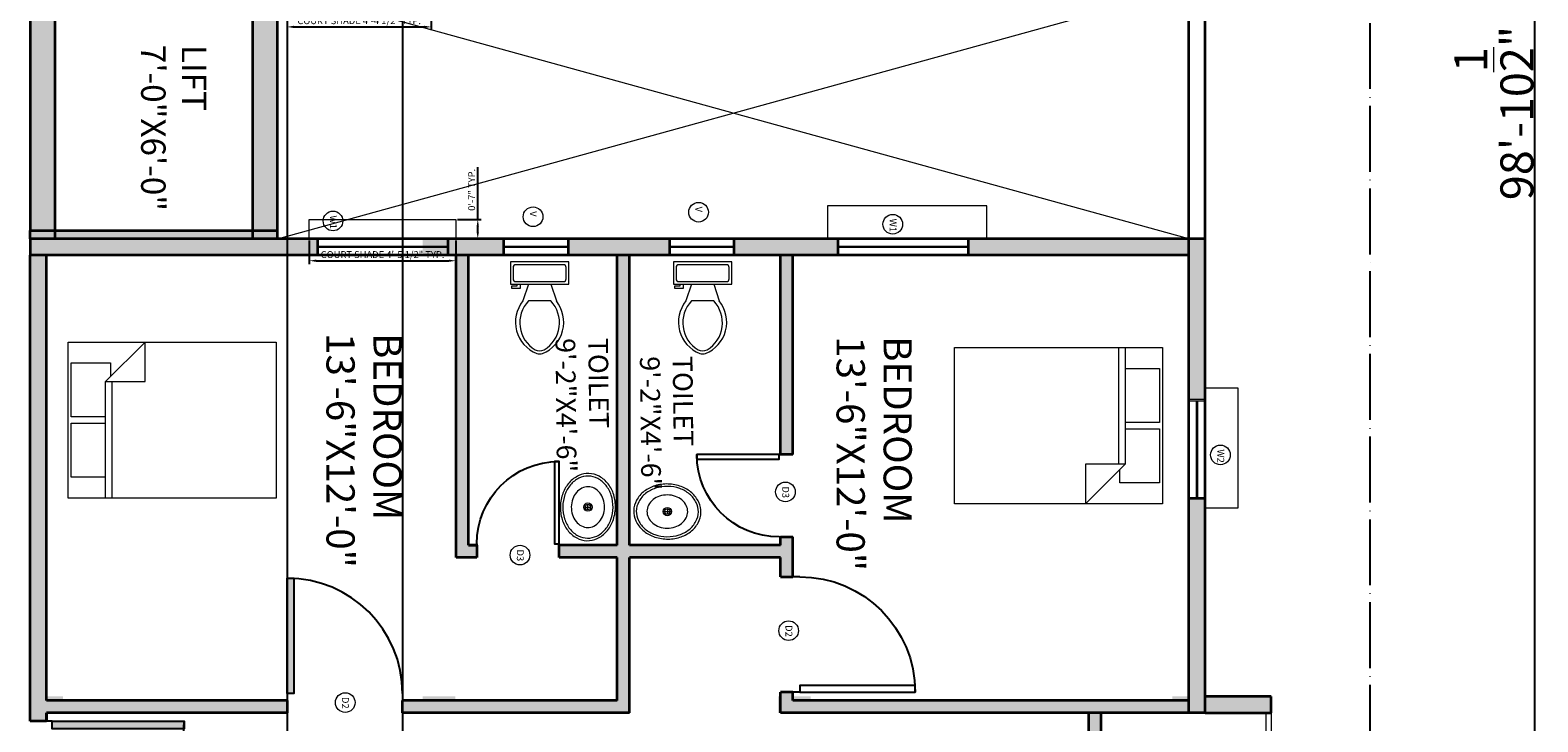
# Model space of a CAD drawing. Units: inches. Extents: x 7028582 to 7030319, y 63109697 to 63111305.
# Tile 13 of 18: x 7029748 to 7030297, y 63110278 to 63110530. Entities that reach past the tile are written whole.
import ezdxf

# ---------------------------------------------------------------- set-up
doc = ezdxf.new("R2010")
doc.units = ezdxf.units.IN
doc.linetypes.add('ACAD_ISO04W100', pattern=[30, 24, -3, 0, -3])
for name, color, linetype, lineweight in [('A-AREA-IDEN', 7, 'Continuous', 18), ('A-DOOR-IDEN', 20, 'Continuous', 13), ('A-FLOR-FIXT', 9, 'Continuous', 18), ('A-FLOR-HRAL', 5, 'Continuous', 18), ('A-FLOR-OPEN', 7, 'Continuous', 13), ('A-GLAZ-IDEN', 20, 'Continuous', 13), ('A-WALL-PATT', 8, 'Continuous', 13), ('C-ANNO-DIMS', 7, 'Continuous', 18), ('C-PROP', 1, 'ACAD_ISO04W100', 25), ('doors', 20, 'Continuous', 25), ('furniture', 9, 'Continuous', 18), ('S-COLS-PATT', 220, 'Continuous', 100), ('walls', 6, 'Continuous', 35), ('WINDOW SHADOW', 9, 'Continuous', 13), ('windows', 5, 'Continuous', 18)]:
    doc.layers.add(name, color=color, linetype=linetype, lineweight=lineweight)
doc.styles.get("Standard").update_dxf_attribs({"font": 'arial.ttf'})
doc.dimstyles.new('ISO-25', dxfattribs={"dimtxt": 2.5, "dimasz": 2.5, "dimexe": 1.25, "dimexo": 0.625, "dimtad": 1, "dimlunit": 4, "dimtxsty": 'Standard', "dimcen": 2.5, "dimadec": 0, "dimazin": 0, "dimtfac": 1, "dimtmove": 0, "dimatfit": 3, "dimfxl": 1, "dimarcsym": 0})

# ---------------------------------------------------------------- blocks, each defined once
blk = doc.blocks.new('*U2')
for p, q in [((0, 0), (0, -5)), ((30, 0), (30, -5))]:
    blk.add_line(p, q)
blk.add_lwpolyline([(0, 0), (0, 30), (1.75, 30), (1.75, 0)], close=True)
blk.add_arc((0, 0), 30, 0, 90)
blk = doc.blocks.new('Toilet - top')
for p, q in [((9.5, -6), (9.5, -2)), ((-10, -8.5), (-8, -8.5)), ((-10, -9.5), (-10, -8.5)), ((-7, -9.5), (-10, -9.5)), ((-8, -8.5), (-8, -8)), ((-7, -8), (-7, -9.5)), ((-4, -8), (-6, -14)), ((4, -8), (6, -14)), ((4, -14), (-4, -14))]:
    blk.add_line(p, q)
blk.add_lwpolyline([(10.5, -8), (10.5, 0), (-10.5, 0), (-10.5, -8)], close=True)
for points in [[(-9.5, -2), (-9.5, -6)], [(8.5, -1), (-8.5, -1)], [(-8.5, -7), (8.5, -7)]]:
    blk.add_lwpolyline(points)
for centre, radius, start, end in [((-8.62, -1.88), 0.884, 81.8699, 188.1301), ((8.62, -1.88), 0.884, 351.8699, 98.1301), ((-8.62, -6.12), 0.884, 171.8699, 278.1301), ((8.62, -6.12), 0.884, 261.8699, 8.1301), ((3.52, -21.58), 12.17, 141.4691, 247.9714), ((4.2, -21.82), 11.33, 136.3677, 238.9468), ((-3.52, -21.58), 12.17, 292.0284, 38.5307), ((-4.2, -21.82), 11.33, 301.053, 43.6321), ((0, -27.88), 4, 245.7318, 294.2682), ((0, -29), 4, 254.8605, 285.1395)]:
    blk.add_arc(centre, radius, start, end)
blk = doc.blocks.new('Sink - Oval top')
for p, q in [((-1, 0), (1, 0)), ((0, 1), (0, -1))]:
    blk.add_line(p, q)
for points in [[(-12.23, 0.39, 0.117634), (-11.46, -3.36, 0.104469), (-8.88, -6.8, 0.090016), (-5.08, -9.07, 0.08192), (-0.32, -10.02, 0.08192), (4.49, -9.38, 0.090016), (8.42, -7.36, 0.104469), (11.22, -4.09, 0.117634), (12.23, -0.39, 0.117634), (11.46, 3.36, 0.104469), (8.88, 6.8, 0.090016), (5.08, 9.07, 0.08192), (0.32, 10.02, 0.08192), (-4.49, 9.38, 0.090016), (-8.42, 7.36, 0.104469), (-11.22, 4.09, 0.117634)], [(-11.29, 0.16, 0.118622), (-10.52, -3.25, 0.104678), (-8.07, -6.36, 0.089562), (-4.54, -8.37, 0.081185), (-0.13, -9.15, 0.081185), (4.3, -8.49, 0.089562), (7.89, -6.58, 0.104678), (10.42, -3.55, 0.118622), (11.29, -0.16, 0.118622), (10.52, 3.25, 0.104678), (8.07, 6.36, 0.089562), (4.54, 8.37, 0.081185), (0.13, 9.15, 0.081185), (-4.3, 8.49, 0.089562), (-7.89, 6.58, 0.104678), (-10.42, 3.55, 0.118622)], [(-7.42, 0.08, 0.118283), (-6.91, -2.17, 0.104607), (-5.29, -4.21, 0.089718), (-2.97, -5.53, 0.081436), (-0.07, -6.04, 0.081436), (2.84, -5.59, 0.089718), (5.2, -4.33, 0.104607), (6.86, -2.32, 0.118283), (7.42, -0.08, 0.118283), (6.91, 2.17, 0.104607), (5.29, 4.21, 0.089718), (2.97, 5.53, 0.081436), (0.07, 6.04, 0.081436), (-2.84, 5.59, 0.089718), (-5.2, 4.33, 0.104607), (-6.86, 2.32, 0.118283)]]:
    blk.add_lwpolyline(points, format="xyb", close=True)
for radius in [1.5, 1]:
    blk.add_circle((0, 0), radius)
blk = doc.blocks.new('Bed - Queen')
for p, q in [((0, -80.00003), (0, 0)), ((0, 0), (59.99999, 0)), ((59.99999, 0), (59.99999, -80.00003)), ((7.99999, -1.2), (28.79998, -1.2)), ((7.99999, -14.4), (7.99999, -1.2)), ((28.79998, -1.2), (28.79998, -14.4)), ((31.19999, -1.2), (51.99999, -1.2)), ((31.19999, -14.4), (31.19999, -1.2)), ((51.99999, -1.2), (51.99999, -16.4)), ((0, -14.4), (44.8, -14.4)), ((44.8, -16.8), (0, -16.8)), ((59.99999, -29.6), (44.8, -14.4)), ((44.8, -14.4), (44.8, -29.6)), ((51.99999, -16.4), (46.79936, -16.4)), ((44.8, -29.6), (59.99999, -29.6)), ((59.99999, -80.00003), (0, -80.00003))]:
    blk.add_line(p, q)
blk = doc.blocks.new('*D10')
at = {"layer": 'C-ANNO-DIMS', "color": 0, "lineweight": -2, "transparency": 16777216}
for p, q in [((7030236.33, 63111093.06), (7030296.71, 63111093.06)), ((7030295.46, 63111090.56), (7030295.46, 63109909.06)), ((7030236.33, 63109906.56), (7030296.71, 63109906.56))]:
    blk.add_line(p, q, dxfattribs=at)
at = {"layer": 'C-ANNO-DIMS', "color": 0, "lineweight": 100, "transparency": 16777216}
for points in [[(7030295.04, 63111090.56), (7030295.88, 63111090.56), (7030295.46, 63111093.06)], [(7030295.04, 63109909.06), (7030295.88, 63109909.06), (7030295.46, 63109906.56)]]:
    blk.add_solid(points, dxfattribs=at)
at = {"layer": 'Defpoints', "color": 0, "lineweight": 100, "transparency": 16777216}
for p in [(7030235.71, 63111093.06), (7030235.71, 63109906.56), (7030295.46, 63109906.56)]:
    blk.add_point(p, dxfattribs=at)
at = {"layer": 'C-ANNO-DIMS', "color": 0, "transparency": 16777216, "insert": (7030280.69, 63110499.81), "char_height": 12, "attachment_point": 5, "rotation": 90}
blk.add_mtext('98\'-10{\\H1x;\\S1/2;}"', dxfattribs=at)
blk = doc.blocks.new('WIN-SASH-36')
for p, q in [((0, 36.05), (0, 0)), ((6, 35.55), (0, 35.55)), ((2.8, 35.55), (2.8, 0.5)), ((3.2, 35.55), (3.2, 0.5)), ((6, 0), (6, 36.05)), ((0, 0.5), (6, 0.5))]:
    blk.add_line(p, q)
blk = doc.blocks.new('WIN-SASH-24')
for p, q in [((24.05, 6), (0, 6)), ((0.5, 6), (0.5, 0)), ((23.55, 0), (23.55, 6)), ((0, 0), (24.05, 0)), ((23.55, 3.2), (0.5, 3.2)), ((23.55, 2.8), (0.5, 2.8))]:
    blk.add_line(p, q)
blk = doc.blocks.new('WIN-SASH-48')
for p, q in [((48.05, 6), (0, 6)), ((0.5, 6), (0.5, 0)), ((47.55, 0), (47.55, 6)), ((47.55, 3.2), (0.5, 3.2)), ((47.55, 2.8), (0.5, 2.8)), ((0, 0), (48.05, 0))]:
    blk.add_line(p, q)
blk = doc.blocks.new('WINDOW-SHADE-SIDE-44')
for p, q in [((12, 43.55), (0, 43.55)), ((12, 0), (12, 43.55)), ((0, 0), (12, 0))]:
    blk.add_line(p, q)
blk = doc.blocks.new('WINDOW-SHADE-HEAD-58')
for p, q in [((57.96, 12), (0, 12)), ((0, 12), (0, 0)), ((57.96, 0), (57.96, 12))]:
    blk.add_line(p, q)
blk = doc.blocks.new('WINDOW-SHADE-COURT-53')
for p, q in [((0, 0), (0, 7.06)), ((0, 7.06), (53.29, 7.06)), ((53.29, 7.06), (53.29, 0))]:
    blk.add_line(p, q)
blk = doc.blocks.new('BALCONY-GUARD-12FT')
for p, q in [((0, 144), (0, 0)), ((2, 144), (2, 0))]:
    blk.add_line(p, q)
blk = doc.blocks.new('TAG-D2-MT-R')
blk.add_circle((3.58, 3.58), 3.58)
at = {"insert": (4.93, 5.6), "char_height": 2.5, "attachment_point": 1, "rotation": 270}
blk.add_mtext_dynamic_manual_height_columns('D2', width=2.5021, gutter_width=12.5, heights=[0], dxfattribs=at)
blk = doc.blocks.new('TAG-D3-MT-R')
blk.add_circle((3.58, 3.58), 3.58)
at = {"insert": (4.93, 5.6), "char_height": 2.5, "attachment_point": 1, "rotation": 270}
blk.add_mtext_dynamic_manual_height_columns('D3', width=2.5021, gutter_width=12.5, heights=[0], dxfattribs=at)
blk = doc.blocks.new('TAG-V-MT-R')
blk.add_circle((3.58, 3.58), 3.58)
at = {"insert": (4.93, 5.6), "char_height": 2.5, "attachment_point": 1, "rotation": 270}
blk.add_mtext_dynamic_manual_height_columns('V', width=2.5021, gutter_width=12.5, heights=[0], dxfattribs=at)
blk = doc.blocks.new('TAG-W1-MT-R')
blk.add_circle((3.58, 3.58), 3.58)
at = {"insert": (4.93, 5.6), "char_height": 2.5, "attachment_point": 1, "rotation": 270}
blk.add_mtext_dynamic_manual_height_columns('W1', width=2.5021, gutter_width=12.5, heights=[0], dxfattribs=at)
blk = doc.blocks.new('TAG-W2-MT-R')
blk.add_circle((3.58, 3.58), 3.58)
at = {"insert": (4.93, 5.6), "char_height": 2.5, "attachment_point": 1, "rotation": 270}
blk.add_mtext_dynamic_manual_height_columns('W2', width=2.5021, gutter_width=12.5, heights=[0], dxfattribs=at)
blk = doc.blocks.new('*D95')
at = {"layer": 'C-ANNO-DIMS', "color": 0, "lineweight": -2, "transparency": 16777216}
for p, q in [((7029841.67, 63110538.39), (7029841.67, 63110529.9)), ((7029894.13, 63110538.39), (7029894.13, 63110529.9)), ((7029844.17, 63110531.15), (7029891.63, 63110531.15))]:
    blk.add_line(p, q, dxfattribs=at)
at = {"layer": 'C-ANNO-DIMS', "color": 0, "lineweight": 100, "transparency": 16777216}
for points in [[(7029844.17, 63110531.56), (7029844.17, 63110530.73), (7029841.67, 63110531.15)], [(7029891.63, 63110531.56), (7029891.63, 63110530.73), (7029894.13, 63110531.15)]]:
    blk.add_solid(points, dxfattribs=at)
at = {"layer": 'Defpoints', "color": 0, "lineweight": 100, "transparency": 16777216}
for p in [(7029841.67, 63110539.02), (7029894.13, 63110539.02), (7029894.13, 63110531.15)]:
    blk.add_point(p, dxfattribs=at)
at = {"layer": 'C-ANNO-DIMS', "color": 0, "transparency": 16777216, "insert": (7029867.9, 63110533.07), "char_height": 2.5, "attachment_point": 5}
blk.add_mtext('COURT SHADE 4\'-4 1/2" TYP.', dxfattribs=at)
blk = doc.blocks.new('*D97')
at = {"layer": 'C-ANNO-DIMS', "color": 0, "lineweight": -2, "transparency": 16777216}
for p, q in [((7029849.76, 63110453.43), (7029849.76, 63110444.81)), ((7029903.05, 63110453.43), (7029903.05, 63110444.81)), ((7029852.26, 63110446.06), (7029900.55, 63110446.06))]:
    blk.add_line(p, q, dxfattribs=at)
at = {"layer": 'C-ANNO-DIMS', "color": 0, "lineweight": 100, "transparency": 16777216}
for points in [[(7029852.26, 63110446.48), (7029852.26, 63110445.65), (7029849.76, 63110446.06)], [(7029900.55, 63110446.48), (7029900.55, 63110445.65), (7029903.05, 63110446.06)]]:
    blk.add_solid(points, dxfattribs=at)
at = {"layer": 'Defpoints', "color": 0, "lineweight": 100, "transparency": 16777216}
for p in [(7029849.76, 63110454.06), (7029903.05, 63110454.06), (7029903.05, 63110446.06)]:
    blk.add_point(p, dxfattribs=at)
at = {"layer": 'C-ANNO-DIMS', "color": 0, "transparency": 16777216, "insert": (7029876.41, 63110447.98), "char_height": 2.5, "attachment_point": 5}
blk.add_mtext('COURT SHADE 4\'-5 1/2" TYP.', dxfattribs=at)
blk = doc.blocks.new('*D98')
at = {"layer": 'C-ANNO-DIMS', "color": 0, "lineweight": -2, "transparency": 16777216}
for p, q in [((7029911.05, 63110461.12), (7029911.05, 63110480.1)), ((7029903.68, 63110461.12), (7029912.3, 63110461.12)), ((7029911.05, 63110456.56), (7029911.05, 63110458.62)), ((7029903.68, 63110454.06), (7029912.3, 63110454.06))]:
    blk.add_line(p, q, dxfattribs=at)
at = {"layer": 'C-ANNO-DIMS', "color": 0, "lineweight": 100, "transparency": 16777216}
for points in [[(7029910.63, 63110458.62), (7029911.46, 63110458.62), (7029911.05, 63110461.12)], [(7029910.63, 63110456.56), (7029911.46, 63110456.56), (7029911.05, 63110454.06)]]:
    blk.add_solid(points, dxfattribs=at)
at = {"layer": 'Defpoints', "color": 0, "lineweight": 100, "transparency": 16777216}
for p in [(7029903.05, 63110461.12), (7029911.05, 63110461.12), (7029903.05, 63110454.06)]:
    blk.add_point(p, dxfattribs=at)
at = {"layer": 'C-ANNO-DIMS', "color": 0, "transparency": 16777216, "insert": (7029909.15, 63110471.86), "char_height": 2.5, "attachment_point": 5, "rotation": 90}
blk.add_mtext('0\'-7" TYP.', dxfattribs=at)
blk = doc.blocks.new('*D105')
at = {"layer": 'C-ANNO-DIMS', "color": 0, "lineweight": -2, "transparency": 16777216}
for p, q in [((7029841.68, 63110859.93), (7029841.68, 63109697.14)), ((7029883.68, 63110859.93), (7029883.68, 63109697.14)), ((7029844.18, 63109698.39), (7029881.18, 63109698.39))]:
    blk.add_line(p, q, dxfattribs=at)
at = {"layer": 'C-ANNO-DIMS', "color": 0, "lineweight": 100, "transparency": 16777216}
for points in [[(7029844.18, 63109698.8), (7029844.18, 63109697.97), (7029841.68, 63109698.39)], [(7029881.18, 63109698.8), (7029881.18, 63109697.97), (7029883.68, 63109698.39)]]:
    blk.add_solid(points, dxfattribs=at)
at = {"layer": 'Defpoints', "color": 0, "lineweight": 100, "transparency": 16777216}
for p in [(7029841.68, 63110860.56), (7029883.68, 63110860.56), (7029883.68, 63109698.39)]:
    blk.add_point(p, dxfattribs=at)
at = {"layer": 'C-ANNO-DIMS', "color": 0, "transparency": 16777216, "insert": (7029862.68, 63109700.29), "char_height": 2.5, "attachment_point": 5}
blk.add_mtext('3\'-6"', dxfattribs=at)

msp = doc.modelspace()

# ---------------------------------------------------------------- hatches: boundary and pattern name
at = {"layer": 'A-WALL-PATT'}
h = msp.add_hatch(color=256, dxfattribs=at)
h.dxf.hatch_style = 1
h.paths.add_polyline_path([(7029757.205, 63110542.557), (7029748.205, 63110542.557), (7029748.205, 63110457.057), (7029757.205, 63110457.057)])
h = msp.add_hatch(color=256, dxfattribs=at)
h.dxf.hatch_style = 1
h.paths.add_polyline_path([(7029838.205, 63110542.557), (7029829.205, 63110542.557), (7029829.205, 63110457.057), (7029838.205, 63110457.057)])
h = msp.add_hatch(color=256, dxfattribs=at)
h.dxf.hatch_style = 1
h.paths.add_polyline_path([(7029757.205, 63110457.057), (7029748.205, 63110457.057), (7029748.205, 63110454.057), (7029757.205, 63110454.057)])
h = msp.add_hatch(color=256, dxfattribs=at)
h.dxf.hatch_style = 1
h.paths.add_polyline_path([(7029748.205, 63110454.057), (7029748.205, 63110448.057), (7029852.47, 63110448.057), (7029852.47, 63110454.057), (7029825.251, 63110454.057)])
h = msp.add_hatch(color=256, dxfattribs=at)
h.dxf.hatch_style = 1
h.paths.add_polyline_path([(7029852.47, 63110454.057), (7029825.251, 63110454.057), (7029748.205, 63110454.057), (7029748.205, 63110448.057), (7029852.47, 63110448.057)])
h = msp.add_hatch(color=256, dxfattribs=at)
h.dxf.hatch_style = 1
h.paths.add_polyline_path([(7029829.205, 63110457.057), (7029757.205, 63110457.057), (7029757.205, 63110454.057), (7029825.251, 63110454.057), (7029829.205, 63110454.057)])
h = msp.add_hatch(color=256, dxfattribs=at)
h.dxf.hatch_style = 1
h.paths.add_polyline_path([(7029838.205, 63110457.057), (7029829.205, 63110457.057), (7029829.205, 63110454.057), (7029838.205, 63110454.057)])
h = msp.add_hatch(color=256, dxfattribs=at)
h.dxf.hatch_style = 1
h.paths.add_polyline_path([(7029900.518, 63110448.057), (7029920.21, 63110448.057), (7029920.21, 63110454.057), (7029900.518, 63110454.057)])
h = msp.add_hatch(color=256, dxfattribs=at)
h.dxf.hatch_style = 1
h.paths.add_polyline_path([(7029980.53, 63110454.057), (7029944.258, 63110454.057), (7029944.258, 63110448.057), (7029980.53, 63110448.057)])
h = msp.add_hatch(color=256, dxfattribs=at)
h.dxf.hatch_style = 1
h.paths.add_polyline_path([(7030041.813, 63110454.057), (7030004.578, 63110454.057), (7030004.578, 63110448.057), (7030041.813, 63110448.057)])
h.paths.add_polyline_path([(7030025.705, 63110448.057), (7030021.205, 63110448.057), (7030021.205, 63110375.557), (7030025.705, 63110375.557)], flags=0)
h = msp.add_hatch(color=256, dxfattribs=at)
h.dxf.hatch_style = 1
h.paths.add_polyline_path([(7030175.705, 63110454.057), (7030089.861, 63110454.057), (7030089.861, 63110448.057), (7030169.705, 63110448.057), (7030169.705, 63110395.515), (7030175.705, 63110395.515)])
h = msp.add_hatch(color=256, dxfattribs=at)
h.dxf.hatch_style = 1
h.paths.add_polyline_path([(7029754.205, 63110278.557), (7029756.205, 63110278.557), (7029804.205, 63110278.557), (7029804.205, 63110275.757), (7029756.205, 63110275.757), (7029756.205, 63110278.557), (7029748.205, 63110278.557), (7029748.205, 63110448.057), (7029754.205, 63110448.057), (7029754.205, 63110286.057), (7029841.685, 63110286.057), (7029841.685, 63110288.557), (7029841.685, 63110330.557), (7029844.135, 63110330.557), (7029844.135, 63110288.557), (7029841.685, 63110288.557), (7029841.685, 63110281.557), (7029754.205, 63110281.557)])
h = msp.add_hatch(color=256, dxfattribs=at)
h.dxf.hatch_style = 1
h.paths.add_polyline_path([(7030025.705, 63110448.057), (7030021.205, 63110448.057), (7030021.205, 63110375.557), (7030025.705, 63110375.557)], flags=0)
h.paths.add_polyline_path([(7030025.705, 63110345.557), (7030021.205, 63110345.557), (7030021.205, 63110342.557), (7029966.205, 63110342.557), (7029966.205, 63110448.057), (7029961.705, 63110448.057), (7029961.705, 63110342.557), (7029940.705, 63110342.557), (7029940.705, 63110338.057), (7029961.705, 63110338.057), (7029961.705, 63110286.057), (7029883.685, 63110286.057), (7029883.685, 63110281.557), (7029966.205, 63110281.557), (7029966.205, 63110338.057), (7030021.205, 63110338.057), (7030021.205, 63110331.057), (7030025.705, 63110331.057)])
h = msp.add_hatch(color=256, dxfattribs=at)
h.dxf.hatch_style = 1
h.paths.add_polyline_path([(7029907.705, 63110448.057), (7029903.205, 63110448.057), (7029903.205, 63110338.057), (7029910.705, 63110338.057), (7029910.705, 63110342.557), (7029907.705, 63110342.557)], flags=17)
h = msp.add_hatch(color=256, dxfattribs=at)
h.dxf.hatch_style = 1
h.paths.add_polyline_path([(7030025.705, 63110448.057), (7030021.205, 63110448.057), (7030021.205, 63110375.557), (7030025.705, 63110375.557)])
h = msp.add_hatch(color=256, dxfattribs=at)
h.dxf.hatch_style = 1
h.paths.add_polyline_path([(7030175.705, 63110359.466), (7030169.705, 63110359.466), (7030169.705, 63110281.557), (7030175.705, 63110281.557)])
h = msp.add_hatch(color=256, dxfattribs=at)
h.dxf.hatch_style = 1
h.paths.add_polyline_path([(7030169.705, 63110286.057), (7030025.705, 63110286.057), (7030025.705, 63110289.057), (7030021.205, 63110289.057), (7030021.205, 63110281.557), (7030169.705, 63110281.557)])
h = msp.add_hatch(color=256, dxfattribs=at)
h.dxf.hatch_style = 1
h.paths.add_polyline_path([(7030199.705, 63110287.557), (7030175.705, 63110287.557), (7030175.705, 63110281.557), (7030199.705, 63110281.557)])
h = msp.add_hatch(color=256, dxfattribs=at)
h.dxf.hatch_style = 1
h.paths.add_polyline_path([(7030137.705, 63110281.557), (7030133.205, 63110281.557), (7030133.205, 63110243.163), (7030137.705, 63110243.163)])
at = {"layer": 'S-COLS-PATT'}
h = msp.add_hatch(color=256, dxfattribs=at)
h.dxf.hatch_style = 1
h.paths.add_polyline_path([(7029760.108, 63110454.057), (7029748.205, 63110454.057), (7029748.205, 63110448.057), (7029760.108, 63110448.057)])
h = msp.add_hatch(color=256, dxfattribs=at)
h.dxf.hatch_style = 1
h.paths.add_polyline_path([(7029902.915, 63110454.057), (7029891, 63110454.057), (7029891, 63110448.057), (7029902.915, 63110448.057)])
h = msp.add_hatch(color=256, dxfattribs=at)
h.dxf.hatch_style = 1
h.paths.add_polyline_path([(7030032.194, 63110454.057), (7030020.279, 63110454.057), (7030020.279, 63110448.057), (7030032.194, 63110448.057)])
h = msp.add_hatch(color=256, dxfattribs=at)
h.dxf.hatch_style = 1
h.paths.add_polyline_path([(7030175.705, 63110454.057), (7030163.791, 63110454.057), (7030163.791, 63110448.057), (7030175.705, 63110448.057)])
h = msp.add_hatch(color=256, dxfattribs=at)
h.dxf.hatch_style = 1
h.paths.add_polyline_path([(7029760.108, 63110287.557), (7029748.205, 63110287.557), (7029748.205, 63110281.557), (7029760.108, 63110281.557)])
h = msp.add_hatch(color=256, dxfattribs=at)
h.dxf.hatch_style = 1
h.paths.add_polyline_path([(7029902.915, 63110287.557), (7029891, 63110287.557), (7029891, 63110281.557), (7029902.915, 63110281.557)])
h = msp.add_hatch(color=256, dxfattribs=at)
h.dxf.hatch_style = 1
h.paths.add_polyline_path([(7030032.194, 63110287.557), (7030020.279, 63110287.557), (7030020.279, 63110281.557), (7030032.194, 63110281.557)])
h = msp.add_hatch(color=256, dxfattribs=at)
h.dxf.hatch_style = 1
h.paths.add_polyline_path([(7030175.705, 63110287.557), (7030163.791, 63110287.557), (7030163.791, 63110281.557), (7030175.705, 63110281.557)])

# ---------------------------------------------------------------- linework, layer by layer
at = {"layer": 'A-FLOR-OPEN'}
for p, q in [((7030169.705, 63110454.057), (7029838.205, 63110545.557)), ((7029838.205, 63110454.057), (7030169.705, 63110545.557))]:
    msp.add_line(p, q, dxfattribs=at)
at = {"layer": 'C-PROP'}
msp.add_line((7030235.705, 63109906.557), (7030235.705, 63111093.057), dxfattribs=at)
at = {"layer": 'walls'}
for p, q in [((7030175.705, 63110281.557), (7030175.705, 63110716.557)), ((7029748.205, 63110542.557), (7029748.205, 63110457.057)), ((7029757.205, 63110545.557), (7029757.205, 63110454.057)), ((7029829.205, 63110454.057), (7029829.205, 63110545.557)), ((7029838.205, 63110454.057), (7029838.205, 63110545.557)), ((7030169.705, 63110281.557), (7030169.705, 63110545.557)), ((7029748.205, 63110454.057), (7029748.205, 63110457.057)), ((7029748.205, 63110457.057), (7029757.205, 63110457.057)), ((7029825.251, 63110454.057), (7029748.205, 63110454.057)), ((7029748.205, 63110454.057), (7029748.205, 63110448.057)), ((7029757.205, 63110457.057), (7029829.205, 63110457.057)), ((7030175.705, 63110454.057), (7029825.251, 63110454.057)), ((7029829.205, 63110457.057), (7029838.205, 63110457.057)), ((7030175.705, 63110281.557), (7030175.705, 63110454.057)), ((7029748.205, 63110278.557), (7029748.205, 63110448.057)), ((7030169.705, 63110448.057), (7029748.205, 63110448.057)), ((7029754.205, 63110286.057), (7029754.205, 63110448.057)), ((7029903.205, 63110338.057), (7029903.205, 63110448.057)), ((7029907.705, 63110342.557), (7029907.705, 63110448.057)), ((7029961.705, 63110342.557), (7029961.705, 63110448.057)), ((7029966.205, 63110342.557), (7029966.205, 63110448.057)), ((7030021.205, 63110375.557), (7030021.205, 63110448.057)), ((7030025.705, 63110375.557), (7030025.705, 63110448.057)), ((7030169.705, 63110281.557), (7030169.705, 63110448.057)), ((7030025.705, 63110375.557), (7030021.205, 63110375.557)), ((7030021.205, 63110342.557), (7030021.205, 63110345.557)), ((7030021.205, 63110342.557), (7030021.205, 63110345.557)), ((7030021.205, 63110345.557), (7030025.705, 63110345.557)), ((7030025.705, 63110331.057), (7030025.705, 63110345.557)), ((7029910.705, 63110338.057), (7029903.205, 63110338.057)), ((7029910.705, 63110342.557), (7029907.705, 63110342.557)), ((7029907.705, 63110342.557), (7029910.705, 63110342.557)), ((7029910.705, 63110342.557), (7029910.705, 63110338.057)), ((7029961.705, 63110342.557), (7029940.705, 63110342.557)), ((7029940.705, 63110338.057), (7029940.705, 63110342.557)), ((7029961.705, 63110338.057), (7029940.705, 63110338.057)), ((7029961.705, 63110286.057), (7029961.705, 63110338.057)), ((7030021.205, 63110342.557), (7029966.205, 63110342.557)), ((7029966.205, 63110281.557), (7029966.205, 63110338.057)), ((7030021.205, 63110338.057), (7029966.205, 63110338.057)), ((7030021.205, 63110331.057), (7030021.205, 63110338.057)), ((7030021.205, 63110331.057), (7030025.705, 63110331.057)), ((7030021.205, 63110281.557), (7030021.205, 63110289.057)), ((7030025.705, 63110289.057), (7030021.205, 63110289.057)), ((7030025.705, 63110286.057), (7030025.705, 63110289.057)), ((7030025.705, 63110286.057), (7030025.705, 63110289.057)), ((7029841.685, 63110286.057), (7029754.205, 63110286.057)), ((7029841.685, 63110286.057), (7029841.685, 63110281.557)), ((7029883.685, 63110281.557), (7029883.685, 63110286.057)), ((7029961.705, 63110286.057), (7029883.685, 63110286.057)), ((7030169.705, 63110286.057), (7030025.705, 63110286.057)), ((7030199.705, 63110287.557), (7030175.705, 63110287.557)), ((7030199.705, 63110281.557), (7030199.705, 63110287.557)), ((7029754.205, 63110278.557), (7029748.205, 63110278.557)), ((7029754.205, 63110278.557), (7029754.205, 63110281.557)), ((7029841.685, 63110281.557), (7029754.205, 63110281.557)), ((7029754.205, 63110281.557), (7029754.205, 63110278.557)), ((7029966.205, 63110281.557), (7029883.685, 63110281.557)), ((7030175.705, 63110281.557), (7030021.205, 63110281.557)), ((7030133.205, 63110281.557), (7030133.205, 63110137.557)), ((7030137.705, 63110281.557), (7030137.705, 63110137.557)), ((7030175.705, 63110281.557), (7030199.705, 63110281.557))]:
    msp.add_line(p, q, dxfattribs=at)
at = {"layer": 'windows'}
for p, q in [((7029852.47, 63110454.057), (7029852.47, 63110448.057)), ((7029900.518, 63110448.057), (7029900.518, 63110454.057)), ((7029920.21, 63110454.057), (7029920.21, 63110448.057)), ((7029944.258, 63110448.057), (7029944.258, 63110454.057)), ((7029980.53, 63110454.057), (7029980.53, 63110448.057)), ((7030004.578, 63110448.057), (7030004.578, 63110454.057)), ((7030041.813, 63110454.057), (7030041.813, 63110448.057)), ((7030089.861, 63110448.057), (7030089.861, 63110454.057)), ((7030175.776, 63110395.515), (7030169.776, 63110395.515)), ((7030169.776, 63110359.466), (7030175.776, 63110359.466))]:
    msp.add_line(p, q, dxfattribs=at)

# ---------------------------------------------------------------- block references
at = {"layer": 'A-DOOR-IDEN'}
for name, p in [('TAG-D3-MT-R', (7030019.402, 63110358.359)), ('TAG-D3-MT-R', (7029922.838, 63110335.381)), ('TAG-D2-MT-R', (7030020.567, 63110307.879)), ('TAG-D2-MT-R', (7029859.234, 63110281.722))]:
    msp.add_blockref(name, p, dxfattribs=at)
at = {"layer": 'A-FLOR-FIXT', "xscale": 1.013555723357934, "yscale": 1.013555723357934, "zscale": 1.013555723357934}
for p in [(7029933.551, 63110445.605), (7029992.842, 63110445.605)]:
    msp.add_blockref('Toilet - top', p, dxfattribs=at)
at = {"layer": 'A-FLOR-FIXT', "rotation": 90}
msp.add_blockref('Sink - Oval top', (7029951.122, 63110356.416), dxfattribs=at)
at = {"layer": 'A-FLOR-FIXT'}
msp.add_blockref('Sink - Oval top', (7029980.015, 63110354.801), dxfattribs=at)
at = {"layer": 'A-FLOR-HRAL'}
msp.add_blockref('BALCONY-GUARD-12FT', (7030197.705, 63110137.557), dxfattribs=at)
at = {"layer": 'A-GLAZ-IDEN'}
for name, p in [('TAG-W1-MT-R', (7029854.806, 63110456.953)), ('TAG-V-MT-R', (7029927.584, 63110458.489)), ('TAG-V-MT-R', (7029987.808, 63110460.151)), ('TAG-W1-MT-R', (7030058.467, 63110455.779)), ('TAG-W2-MT-R', (7030177.672, 63110371.827))]:
    msp.add_blockref(name, p, dxfattribs=at)
at = {"layer": 'doors', "xscale": -1}
msp.add_blockref('*U2', (7029940.705, 63110343.057), dxfattribs=at)
at = {"layer": 'doors', "xscale": -1, "rotation": 90}
msp.add_blockref('*U2', (7030020.705, 63110375.557), dxfattribs=at)
at = {"layer": 'doors', "xscale": 1.399999999999999, "yscale": 1.399999999999999, "zscale": 1.399999999999999}
msp.add_blockref('*U2', (7029841.685, 63110288.557), dxfattribs=at)
at = {"layer": 'doors', "rotation": 270}
for p, xscale, yscale, zscale in [((7030028.205, 63110289.057), -1.399999999999999, 1.399999999999999, 1.399999999999999), ((7029756.205, 63110278.557), 1.599999999999999, 1.599999999999999, 1.599999999999999)]:
    msp.add_blockref('*U2', p, dxfattribs=dict(at, xscale=xscale, yscale=yscale, zscale=zscale))
at = {"layer": 'furniture', "xscale": 0.9464141645025947, "yscale": 0.9464141645025947, "zscale": 0.9464141645025947}
for p, rotation in [((7029761.974, 63110359.688), 89.99999999999999), ((7030160.206, 63110414.435), 270)]:
    msp.add_blockref('Bed - Queen', p, dxfattribs=dict(at, rotation=rotation))
at = {"layer": 'WINDOW SHADOW'}
for name, p in [('WINDOW-SHADE-HEAD-58', (7030038.324, 63110454.057)), ('WINDOW-SHADE-COURT-53', (7029849.762, 63110454.057)), ('WINDOW-SHADE-SIDE-44', (7030175.705, 63110356.171))]:
    msp.add_blockref(name, p, dxfattribs=at)
at = {"layer": 'windows'}
for name, p in [('WIN-SASH-48', (7029852.47, 63110448.057)), ('WIN-SASH-24', (7029920.21, 63110448.057)), ('WIN-SASH-24', (7029980.53, 63110448.057)), ('WIN-SASH-48', (7030041.813, 63110448.057))]:
    msp.add_blockref(name, p, dxfattribs=at)
at = {"layer": 'windows', "rotation": 180}
msp.add_blockref('WIN-SASH-36', (7030175.776, 63110395.515), dxfattribs=at)

# ---------------------------------------------------------------- texts
at = {"layer": 'A-AREA-IDEN', "attachment_point": 1}
for s, width, gutter_width, insert, char_height, rotation in [('LIFT\\P7\'-0"X6\'-0"', 27.37587, 44.409, (7029812.273, 63110524.612), 8.88185, 270), ('BEDROOM\\P13\'-6"X12\'-0"', 82.04322, 51.315, (7029883.378, 63110419.737), 10.26307, 270), ('TOILET\\P9\'-2"X4\'-6"', 42.97461, 35.821, (7029958.409, 63110418.065), 7.16426, 270.6464), ('BEDROOM\\P13\'-6"X12\'-0"', 82.04322, 51.315, (7030068.956, 63110418.575), 10.26307, 270), ('TOILET\\P9\'-2"X4\'-6"', 42.97461, 35.821, (7029989.133, 63110411.477), 7.16426, 270.6464)]:
    msp.add_mtext_dynamic_manual_height_columns(s, width=width, gutter_width=gutter_width, heights=[0], dxfattribs=dict(at, insert=insert, char_height=char_height, rotation=rotation))

# ---------------------------------------------------------------- dimensions: what is measured, and where the dimension line sits
at = {"layer": 'C-ANNO-DIMS'}
dim = msp.add_linear_dim(base=(7030295.462, 63109906.557), p1=(7030235.705, 63111093.057), p2=(7030235.705, 63109906.557), angle=90, dimstyle='ISO-25', override={"dimtxt": 12, "dimclrd": 0, "dimclre": 0, "dimclrt": 0}, dxfattribs=at)
dim.commit()
dim.dimension.update_dxf_attribs({"geometry": '*D10', "text_midpoint": (7030280.685, 63110499.807)})
dim = msp.add_linear_dim(base=(7029883.685, 63109698.385), p1=(7029841.685, 63110860.557), p2=(7029883.685, 63110860.557), dimstyle='ISO-25', override={"dimdec": 1, "dimlfac": 1, "dimrnd": 0, "dimzin": 1, "dimdsep": 46, "dimlunit": 4, "dimfrac": 2}, dxfattribs=at)
dim.commit()
dim.dimension.update_dxf_attribs({"geometry": '*D105', "text_midpoint": (7029862.685, 63109700.288)})
for base, p1, p2, picture, middle in [((7029894.126, 63110531.148), (7029841.671, 63110539.016), (7029894.126, 63110539.016), '*D95', (7029867.898, 63110533.067)), ((7029903.054, 63110446.063), (7029849.762, 63110454.057), (7029903.054, 63110454.057), '*D97', (7029876.408, 63110447.981))]:
    dim = msp.add_linear_dim(base=base, p1=p1, p2=p2, text='COURT SHADE <> TYP.', dimstyle='ISO-25', override={"dimdec": 1, "dimlfac": 1, "dimrnd": 0, "dimzin": 1, "dimdsep": 46, "dimlunit": 4, "dimfrac": 2}, dxfattribs=at)
    dim.commit()
    dim.dimension.update_dxf_attribs({"geometry": picture, "text_midpoint": middle})
dim = msp.add_linear_dim(base=(7029911.048, 63110461.115), p1=(7029903.054, 63110454.057), p2=(7029903.054, 63110461.115), angle=90, text='<> TYP.', dimstyle='ISO-25', override={"dimdec": 1, "dimlfac": 1, "dimrnd": 0, "dimzin": 1, "dimdsep": 46, "dimlunit": 4, "dimfrac": 2}, dxfattribs=at)
dim.commit()
dim.dimension.update_dxf_attribs({"geometry": '*D98', "text_midpoint": (7029909.147, 63110471.86)})

doc.saveas('drawing.dxf')
